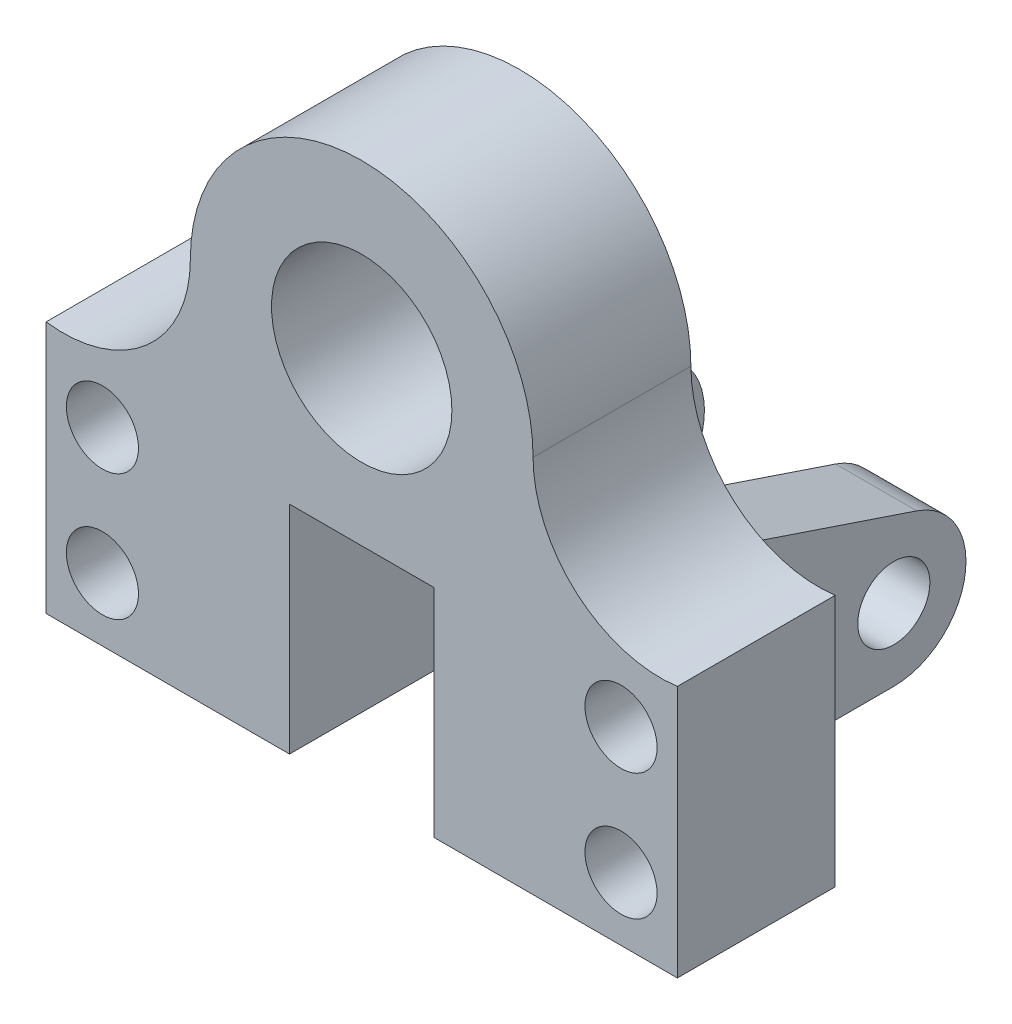
ISO-10303-21;
HEADER;
FILE_DESCRIPTION(('STEP AP214'),'2;1');
FILE_NAME('part.step','',(''),(''),'','','');
FILE_SCHEMA(('AUTOMOTIVE_DESIGN { 1 0 10303 214 1 1 1 1 }'));
ENDSEC;
DATA;
#1=APPLICATION_CONTEXT('core data for automotive mechanical design processes');
#2=APPLICATION_PROTOCOL_DEFINITION('international standard','automotive_design',2000,#1);
#3=PRODUCT_CONTEXT('',#1,'mechanical');
#4=PRODUCT('Part','Part','',(#3));
#5=PRODUCT_RELATED_PRODUCT_CATEGORY('part','',(#4));
#6=PRODUCT_DEFINITION_FORMATION('','',#4);
#7=PRODUCT_DEFINITION_CONTEXT('part definition',#1,'design');
#8=PRODUCT_DEFINITION('design','',#6,#7);
#9=PRODUCT_DEFINITION_SHAPE('','',#8);
#10=(LENGTH_UNIT() NAMED_UNIT(*) SI_UNIT(.MILLI.,.METRE.));
#11=(NAMED_UNIT(*) PLANE_ANGLE_UNIT() SI_UNIT($,.RADIAN.));
#12=(NAMED_UNIT(*) SI_UNIT($,.STERADIAN.) SOLID_ANGLE_UNIT());
#13=UNCERTAINTY_MEASURE_WITH_UNIT(LENGTH_MEASURE(1.E-05),#10,'distance_accuracy_value','');
#14=(GEOMETRIC_REPRESENTATION_CONTEXT(3) GLOBAL_UNCERTAINTY_ASSIGNED_CONTEXT((#13)) GLOBAL_UNIT_ASSIGNED_CONTEXT((#10,
#11,#12)) REPRESENTATION_CONTEXT('',''));
#15=CARTESIAN_POINT('',(0.,0.,0.));
#16=DIRECTION('',(0.,0.,1.));
#17=DIRECTION('',(1.,0.,0.));
#18=AXIS2_PLACEMENT_3D('',#15,#16,#17);
#19=CARTESIAN_POINT('',(-70.,-84.,35.));
#20=DIRECTION('',(0.,1.,0.));
#21=DIRECTION('',(0.,0.,1.));
#22=AXIS2_PLACEMENT_3D('',#19,#20,#21);
#23=PLANE('',#22);
#24=DIRECTION('',(0.,0.,-1.));
#25=VECTOR('',#24,1.);
#26=CARTESIAN_POINT('',(-16.,-84.,35.));
#27=LINE('',#26,#25);
#28=CARTESIAN_POINT('',(-16.,-84.,35.));
#29=VERTEX_POINT('',#28);
#30=CARTESIAN_POINT('',(-16.,-84.,0.));
#31=VERTEX_POINT('',#30);
#32=EDGE_CURVE('E175',#29,#31,#27,.T.);
#33=ORIENTED_EDGE('',*,*,#32,.F.);
#34=DIRECTION('',(1.,0.,0.));
#35=VECTOR('',#34,1.);
#36=CARTESIAN_POINT('',(-70.,-84.,35.));
#37=LINE('',#36,#35);
#38=CARTESIAN_POINT('',(-70.,-84.,35.));
#39=VERTEX_POINT('',#38);
#40=EDGE_CURVE('E189',#39,#29,#37,.T.);
#41=ORIENTED_EDGE('',*,*,#40,.F.);
#42=DIRECTION('',(0.,0.,-1.));
#43=VECTOR('',#42,1.);
#44=CARTESIAN_POINT('',(-70.,-84.,35.));
#45=LINE('',#44,#43);
#46=CARTESIAN_POINT('',(-70.,-84.,0.));
#47=VERTEX_POINT('',#46);
#48=EDGE_CURVE('E231',#39,#47,#45,.T.);
#49=ORIENTED_EDGE('',*,*,#48,.T.);
#50=DIRECTION('',(1.,0.,0.));
#51=VECTOR('',#50,1.);
#52=CARTESIAN_POINT('',(-70.,-84.,0.));
#53=LINE('',#52,#51);
#54=CARTESIAN_POINT('',(-38.,-84.,0.));
#55=VERTEX_POINT('',#54);
#56=EDGE_CURVE('E211',#47,#55,#53,.T.);
#57=ORIENTED_EDGE('',*,*,#56,.T.);
#58=DIRECTION('',(0.,0.,-1.));
#59=VECTOR('',#58,1.);
#60=CARTESIAN_POINT('',(-38.,-84.,0.));
#61=LINE('',#60,#59);
#62=CARTESIAN_POINT('',(-38.,-84.,-45.));
#63=VERTEX_POINT('',#62);
#64=EDGE_CURVE('E292',#55,#63,#61,.T.);
#65=ORIENTED_EDGE('',*,*,#64,.T.);
#66=DIRECTION('',(-1.,0.,0.));
#67=VECTOR('',#66,1.);
#68=CARTESIAN_POINT('',(-20.,-84.,-45.));
#69=LINE('',#68,#67);
#70=CARTESIAN_POINT('',(-20.,-84.,-45.));
#71=VERTEX_POINT('',#70);
#72=EDGE_CURVE('E304',#71,#63,#69,.T.);
#73=ORIENTED_EDGE('',*,*,#72,.F.);
#74=DIRECTION('',(0.,0.,-1.));
#75=VECTOR('',#74,1.);
#76=CARTESIAN_POINT('',(-20.,-84.,0.));
#77=LINE('',#76,#75);
#78=CARTESIAN_POINT('',(-20.,-84.,0.));
#79=VERTEX_POINT('',#78);
#80=EDGE_CURVE('E386',#79,#71,#77,.T.);
#81=ORIENTED_EDGE('',*,*,#80,.F.);
#82=EDGE_CURVE('E214',#79,#31,#53,.T.);
#83=ORIENTED_EDGE('',*,*,#82,.T.);
#84=EDGE_LOOP('',(#33,#41,#49,#57,#65,#73,#81,#83));
#85=FACE_BOUND('',#84,.T.);
#86=ADVANCED_FACE('F41',(#85),#23,.F.);
#87=CARTESIAN_POINT('',(-66.25,0.,0.));
#88=DIRECTION('',(0.,0.,1.));
#89=DIRECTION('',(1.,0.,0.));
#90=AXIS2_PLACEMENT_3D('',#87,#88,#89);
#91=PLANE('',#90);
#92=CARTESIAN_POINT('',(0.,0.,0.));
#93=DIRECTION('',(0.,0.,1.));
#94=DIRECTION('',(1.,0.,0.));
#95=AXIS2_PLACEMENT_3D('',#92,#93,#94);
#96=CIRCLE('',#95,21.);
#97=CARTESIAN_POINT('',(21.,0.,0.));
#98=VERTEX_POINT('',#97);
#99=EDGE_CURVE('E49',#98,#98,#96,.T.);
#100=ORIENTED_EDGE('',*,*,#99,.T.);
#101=EDGE_LOOP('',(#100));
#102=FACE_BOUND('',#101,.T.);
#103=CARTESIAN_POINT('',(-57.5,-70.,0.));
#104=DIRECTION('',(0.,0.,1.));
#105=DIRECTION('',(1.,0.,0.));
#106=AXIS2_PLACEMENT_3D('',#103,#104,#105);
#107=CIRCLE('',#106,8.);
#108=CARTESIAN_POINT('',(-49.5,-70.,0.));
#109=VERTEX_POINT('',#108);
#110=EDGE_CURVE('E356',#109,#109,#107,.T.);
#111=ORIENTED_EDGE('',*,*,#110,.T.);
#112=EDGE_LOOP('',(#111));
#113=FACE_BOUND('',#112,.T.);
#114=CARTESIAN_POINT('',(57.5,-42.,0.));
#115=DIRECTION('',(0.,0.,1.));
#116=DIRECTION('',(1.,0.,0.));
#117=AXIS2_PLACEMENT_3D('',#114,#115,#116);
#118=CIRCLE('',#117,8.00000000000003);
#119=CARTESIAN_POINT('',(65.5,-42.,0.));
#120=VERTEX_POINT('',#119);
#121=EDGE_CURVE('E349',#120,#120,#118,.T.);
#122=ORIENTED_EDGE('',*,*,#121,.T.);
#123=EDGE_LOOP('',(#122));
#124=FACE_BOUND('',#123,.T.);
#125=CARTESIAN_POINT('',(57.5,-70.,0.));
#126=DIRECTION('',(0.,0.,1.));
#127=DIRECTION('',(1.,0.,0.));
#128=AXIS2_PLACEMENT_3D('',#125,#126,#127);
#129=CIRCLE('',#128,8.00000000000001);
#130=CARTESIAN_POINT('',(65.5,-70.,0.));
#131=VERTEX_POINT('',#130);
#132=EDGE_CURVE('E345',#131,#131,#129,.T.);
#133=ORIENTED_EDGE('',*,*,#132,.T.);
#134=EDGE_LOOP('',(#133));
#135=FACE_BOUND('',#134,.T.);
#136=CARTESIAN_POINT('',(-57.5,-42.,0.));
#137=DIRECTION('',(0.,0.,1.));
#138=DIRECTION('',(1.,0.,0.));
#139=AXIS2_PLACEMENT_3D('',#136,#137,#138);
#140=CIRCLE('',#139,8.);
#141=CARTESIAN_POINT('',(-49.5,-42.,0.));
#142=VERTEX_POINT('',#141);
#143=EDGE_CURVE('E365',#142,#142,#140,.T.);
#144=ORIENTED_EDGE('',*,*,#143,.T.);
#145=EDGE_LOOP('',(#144));
#146=FACE_BOUND('',#145,.T.);
#147=DIRECTION('',(0.,-1.,0.));
#148=VECTOR('',#147,1.);
#149=CARTESIAN_POINT('',(16.,-36.,0.));
#150=LINE('',#149,#148);
#151=CARTESIAN_POINT('',(16.,-36.,0.));
#152=VERTEX_POINT('',#151);
#153=CARTESIAN_POINT('',(16.,-84.,0.));
#154=VERTEX_POINT('',#153);
#155=EDGE_CURVE('E169',#152,#154,#150,.T.);
#156=ORIENTED_EDGE('',*,*,#155,.F.);
#157=DIRECTION('',(1.,0.,0.));
#158=VECTOR('',#157,1.);
#159=CARTESIAN_POINT('',(-16.,-36.,0.));
#160=LINE('',#159,#158);
#161=CARTESIAN_POINT('',(-16.,-36.,0.));
#162=VERTEX_POINT('',#161);
#163=EDGE_CURVE('E181',#162,#152,#160,.T.);
#164=ORIENTED_EDGE('',*,*,#163,.F.);
#165=DIRECTION('',(0.,1.,0.));
#166=VECTOR('',#165,1.);
#167=CARTESIAN_POINT('',(-16.,-84.,0.));
#168=LINE('',#167,#166);
#169=EDGE_CURVE('E396',#31,#162,#168,.T.);
#170=ORIENTED_EDGE('',*,*,#169,.F.);
#171=ORIENTED_EDGE('',*,*,#82,.F.);
#172=DIRECTION('',(0.,-1.,0.));
#173=VECTOR('',#172,1.);
#174=CARTESIAN_POINT('',(-20.,-36.,0.));
#175=LINE('',#174,#173);
#176=CARTESIAN_POINT('',(-20.,-36.,0.));
#177=VERTEX_POINT('',#176);
#178=EDGE_CURVE('E395',#177,#79,#175,.T.);
#179=ORIENTED_EDGE('',*,*,#178,.F.);
#180=DIRECTION('',(-1.,0.,0.));
#181=VECTOR('',#180,1.);
#182=CARTESIAN_POINT('',(-20.,-36.,0.));
#183=LINE('',#182,#181);
#184=CARTESIAN_POINT('',(-38.,-36.,0.));
#185=VERTEX_POINT('',#184);
#186=EDGE_CURVE('E62',#177,#185,#183,.T.);
#187=ORIENTED_EDGE('',*,*,#186,.T.);
#188=DIRECTION('',(0.,-1.,0.));
#189=VECTOR('',#188,1.);
#190=CARTESIAN_POINT('',(-38.,-36.,0.));
#191=LINE('',#190,#189);
#192=EDGE_CURVE('E290',#185,#55,#191,.T.);
#193=ORIENTED_EDGE('',*,*,#192,.T.);
#194=ORIENTED_EDGE('',*,*,#56,.F.);
#195=DIRECTION('',(0.,-1.,0.));
#196=VECTOR('',#195,1.);
#197=CARTESIAN_POINT('',(-70.,-28.,0.));
#198=LINE('',#197,#196);
#199=CARTESIAN_POINT('',(-70.,-28.,0.));
#200=VERTEX_POINT('',#199);
#201=EDGE_CURVE('E210',#200,#47,#198,.T.);
#202=ORIENTED_EDGE('',*,*,#201,.F.);
#203=CARTESIAN_POINT('',(-66.25,0.,0.));
#204=DIRECTION('',(0.,0.,-1.));
#205=DIRECTION('',(1.,0.,0.));
#206=AXIS2_PLACEMENT_3D('',#203,#204,#205);
#207=CIRCLE('',#206,28.25);
#208=CARTESIAN_POINT('',(-38.,0.,0.));
#209=VERTEX_POINT('',#208);
#210=EDGE_CURVE('E204',#209,#200,#207,.T.);
#211=ORIENTED_EDGE('',*,*,#210,.F.);
#212=CARTESIAN_POINT('',(0.,0.,0.));
#213=DIRECTION('',(0.,0.,1.));
#214=DIRECTION('',(1.,0.,0.));
#215=AXIS2_PLACEMENT_3D('',#212,#213,#214);
#216=CIRCLE('',#215,38.);
#217=CARTESIAN_POINT('',(38.,0.,0.));
#218=VERTEX_POINT('',#217);
#219=EDGE_CURVE('E219',#218,#209,#216,.T.);
#220=ORIENTED_EDGE('',*,*,#219,.F.);
#221=CARTESIAN_POINT('',(66.25,0.,0.));
#222=DIRECTION('',(0.,0.,-1.));
#223=DIRECTION('',(1.,0.,0.));
#224=AXIS2_PLACEMENT_3D('',#221,#222,#223);
#225=CIRCLE('',#224,28.25);
#226=CARTESIAN_POINT('',(70.,-28.,0.));
#227=VERTEX_POINT('',#226);
#228=EDGE_CURVE('E217',#227,#218,#225,.T.);
#229=ORIENTED_EDGE('',*,*,#228,.F.);
#230=DIRECTION('',(0.,1.,0.));
#231=VECTOR('',#230,1.);
#232=CARTESIAN_POINT('',(70.,-84.,0.));
#233=LINE('',#232,#231);
#234=CARTESIAN_POINT('',(70.,-84.,0.));
#235=VERTEX_POINT('',#234);
#236=EDGE_CURVE('E212',#235,#227,#233,.T.);
#237=ORIENTED_EDGE('',*,*,#236,.F.);
#238=CARTESIAN_POINT('',(38.,-84.,0.));
#239=VERTEX_POINT('',#238);
#240=EDGE_CURVE('E209',#239,#235,#53,.T.);
#241=ORIENTED_EDGE('',*,*,#240,.F.);
#242=DIRECTION('',(0.,-1.,0.));
#243=VECTOR('',#242,1.);
#244=CARTESIAN_POINT('',(38.,-84.,0.));
#245=LINE('',#244,#243);
#246=CARTESIAN_POINT('',(38.,-36.,0.));
#247=VERTEX_POINT('',#246);
#248=EDGE_CURVE('E321',#247,#239,#245,.T.);
#249=ORIENTED_EDGE('',*,*,#248,.F.);
#250=DIRECTION('',(1.,0.,0.));
#251=VECTOR('',#250,1.);
#252=CARTESIAN_POINT('',(20.,-36.,0.));
#253=LINE('',#252,#251);
#254=CARTESIAN_POINT('',(20.,-36.,0.));
#255=VERTEX_POINT('',#254);
#256=EDGE_CURVE('E337',#255,#247,#253,.T.);
#257=ORIENTED_EDGE('',*,*,#256,.F.);
#258=DIRECTION('',(0.,-1.,0.));
#259=VECTOR('',#258,1.);
#260=CARTESIAN_POINT('',(20.,-84.,0.));
#261=LINE('',#260,#259);
#262=CARTESIAN_POINT('',(20.,-84.,0.));
#263=VERTEX_POINT('',#262);
#264=EDGE_CURVE('E326',#255,#263,#261,.T.);
#265=ORIENTED_EDGE('',*,*,#264,.T.);
#266=EDGE_CURVE('E216',#154,#263,#53,.T.);
#267=ORIENTED_EDGE('',*,*,#266,.F.);
#268=EDGE_LOOP('',(#156,#164,#170,#171,#179,#187,#193,#194,#202,#211,#220,#229,#237,#241,#249,
#257,#265,#267));
#269=FACE_BOUND('',#268,.T.);
#270=ADVANCED_FACE('F239',(#102,#113,#124,#135,#146,#269),#91,.F.);
#271=CARTESIAN_POINT('',(-66.25,0.,35.));
#272=DIRECTION('',(0.,0.,1.));
#273=DIRECTION('',(1.,0.,0.));
#274=AXIS2_PLACEMENT_3D('',#271,#272,#273);
#275=PLANE('',#274);
#276=CARTESIAN_POINT('',(-57.5,-70.,35.));
#277=DIRECTION('',(0.,0.,1.));
#278=DIRECTION('',(1.,0.,0.));
#279=AXIS2_PLACEMENT_3D('',#276,#277,#278);
#280=CIRCLE('',#279,8.);
#281=CARTESIAN_POINT('',(-49.5,-70.,35.));
#282=VERTEX_POINT('',#281);
#283=EDGE_CURVE('E355',#282,#282,#280,.T.);
#284=ORIENTED_EDGE('',*,*,#283,.F.);
#285=EDGE_LOOP('',(#284));
#286=FACE_BOUND('',#285,.T.);
#287=CARTESIAN_POINT('',(57.5,-42.,35.));
#288=DIRECTION('',(0.,0.,1.));
#289=DIRECTION('',(1.,0.,0.));
#290=AXIS2_PLACEMENT_3D('',#287,#288,#289);
#291=CIRCLE('',#290,8.00000000000003);
#292=CARTESIAN_POINT('',(65.5,-42.,35.));
#293=VERTEX_POINT('',#292);
#294=EDGE_CURVE('E357',#293,#293,#291,.T.);
#295=ORIENTED_EDGE('',*,*,#294,.F.);
#296=EDGE_LOOP('',(#295));
#297=FACE_BOUND('',#296,.T.);
#298=CARTESIAN_POINT('',(57.5,-70.,35.));
#299=DIRECTION('',(0.,0.,1.));
#300=DIRECTION('',(1.,0.,0.));
#301=AXIS2_PLACEMENT_3D('',#298,#299,#300);
#302=CIRCLE('',#301,8.00000000000001);
#303=CARTESIAN_POINT('',(65.5,-70.,35.));
#304=VERTEX_POINT('',#303);
#305=EDGE_CURVE('E347',#304,#304,#302,.T.);
#306=ORIENTED_EDGE('',*,*,#305,.F.);
#307=EDGE_LOOP('',(#306));
#308=FACE_BOUND('',#307,.T.);
#309=CARTESIAN_POINT('',(-57.5,-42.,35.));
#310=DIRECTION('',(0.,0.,1.));
#311=DIRECTION('',(1.,0.,0.));
#312=AXIS2_PLACEMENT_3D('',#309,#310,#311);
#313=CIRCLE('',#312,8.);
#314=CARTESIAN_POINT('',(-49.5,-42.,35.));
#315=VERTEX_POINT('',#314);
#316=EDGE_CURVE('E352',#315,#315,#313,.T.);
#317=ORIENTED_EDGE('',*,*,#316,.F.);
#318=EDGE_LOOP('',(#317));
#319=FACE_BOUND('',#318,.T.);
#320=CARTESIAN_POINT('',(0.,0.,35.));
#321=DIRECTION('',(0.,0.,1.));
#322=DIRECTION('',(1.,0.,0.));
#323=AXIS2_PLACEMENT_3D('',#320,#321,#322);
#324=CIRCLE('',#323,20.);
#325=CARTESIAN_POINT('',(20.,0.,35.));
#326=VERTEX_POINT('',#325);
#327=EDGE_CURVE('E208',#326,#326,#324,.T.);
#328=ORIENTED_EDGE('',*,*,#327,.F.);
#329=EDGE_LOOP('',(#328));
#330=FACE_BOUND('',#329,.T.);
#331=DIRECTION('',(1.,0.,0.));
#332=VECTOR('',#331,1.);
#333=CARTESIAN_POINT('',(-16.,-36.,35.));
#334=LINE('',#333,#332);
#335=CARTESIAN_POINT('',(-16.,-36.,35.));
#336=VERTEX_POINT('',#335);
#337=CARTESIAN_POINT('',(16.,-36.,35.));
#338=VERTEX_POINT('',#337);
#339=EDGE_CURVE('E171',#336,#338,#334,.T.);
#340=ORIENTED_EDGE('',*,*,#339,.T.);
#341=DIRECTION('',(0.,-1.,0.));
#342=VECTOR('',#341,1.);
#343=CARTESIAN_POINT('',(16.,-36.,35.));
#344=LINE('',#343,#342);
#345=CARTESIAN_POINT('',(16.,-84.,35.));
#346=VERTEX_POINT('',#345);
#347=EDGE_CURVE('E60',#338,#346,#344,.T.);
#348=ORIENTED_EDGE('',*,*,#347,.T.);
#349=CARTESIAN_POINT('',(70.,-84.,35.));
#350=VERTEX_POINT('',#349);
#351=EDGE_CURVE('E178',#346,#350,#37,.T.);
#352=ORIENTED_EDGE('',*,*,#351,.T.);
#353=DIRECTION('',(0.,1.,0.));
#354=VECTOR('',#353,1.);
#355=CARTESIAN_POINT('',(70.,-84.,35.));
#356=LINE('',#355,#354);
#357=CARTESIAN_POINT('',(70.,-28.,35.));
#358=VERTEX_POINT('',#357);
#359=EDGE_CURVE('E193',#350,#358,#356,.T.);
#360=ORIENTED_EDGE('',*,*,#359,.T.);
#361=CARTESIAN_POINT('',(66.25,0.,35.));
#362=DIRECTION('',(0.,0.,-1.));
#363=DIRECTION('',(1.,0.,0.));
#364=AXIS2_PLACEMENT_3D('',#361,#362,#363);
#365=CIRCLE('',#364,28.25);
#366=CARTESIAN_POINT('',(38.,0.,35.));
#367=VERTEX_POINT('',#366);
#368=EDGE_CURVE('E200',#358,#367,#365,.T.);
#369=ORIENTED_EDGE('',*,*,#368,.T.);
#370=CARTESIAN_POINT('',(0.,0.,35.));
#371=DIRECTION('',(0.,0.,1.));
#372=DIRECTION('',(1.,0.,0.));
#373=AXIS2_PLACEMENT_3D('',#370,#371,#372);
#374=CIRCLE('',#373,38.);
#375=CARTESIAN_POINT('',(-38.,0.,35.));
#376=VERTEX_POINT('',#375);
#377=EDGE_CURVE('E203',#367,#376,#374,.T.);
#378=ORIENTED_EDGE('',*,*,#377,.T.);
#379=CARTESIAN_POINT('',(-66.25,0.,35.));
#380=DIRECTION('',(0.,0.,-1.));
#381=DIRECTION('',(1.,0.,0.));
#382=AXIS2_PLACEMENT_3D('',#379,#380,#381);
#383=CIRCLE('',#382,28.25);
#384=CARTESIAN_POINT('',(-70.,-28.,35.));
#385=VERTEX_POINT('',#384);
#386=EDGE_CURVE('E192',#376,#385,#383,.T.);
#387=ORIENTED_EDGE('',*,*,#386,.T.);
#388=DIRECTION('',(0.,-1.,0.));
#389=VECTOR('',#388,1.);
#390=CARTESIAN_POINT('',(-70.,-28.,35.));
#391=LINE('',#390,#389);
#392=EDGE_CURVE('E187',#385,#39,#391,.T.);
#393=ORIENTED_EDGE('',*,*,#392,.T.);
#394=ORIENTED_EDGE('',*,*,#40,.T.);
#395=DIRECTION('',(0.,1.,0.));
#396=VECTOR('',#395,1.);
#397=CARTESIAN_POINT('',(-16.,-84.,35.));
#398=LINE('',#397,#396);
#399=EDGE_CURVE('E185',#29,#336,#398,.T.);
#400=ORIENTED_EDGE('',*,*,#399,.T.);
#401=EDGE_LOOP('',(#340,#348,#352,#360,#369,#378,#387,#393,#394,#400));
#402=FACE_BOUND('',#401,.T.);
#403=ADVANCED_FACE('F180',(#286,#297,#308,#319,#330,#402),#275,.T.);
#404=CARTESIAN_POINT('',(-66.25,0.,35.));
#405=DIRECTION('',(0.,0.,-1.));
#406=DIRECTION('',(-1.,0.,0.));
#407=AXIS2_PLACEMENT_3D('',#404,#405,#406);
#408=CYLINDRICAL_SURFACE('',#407,28.25);
#409=ORIENTED_EDGE('',*,*,#210,.T.);
#410=DIRECTION('',(0.,0.,-1.));
#411=VECTOR('',#410,1.);
#412=CARTESIAN_POINT('',(-70.,-28.,35.));
#413=LINE('',#412,#411);
#414=EDGE_CURVE('E232',#385,#200,#413,.T.);
#415=ORIENTED_EDGE('',*,*,#414,.F.);
#416=ORIENTED_EDGE('',*,*,#386,.F.);
#417=DIRECTION('',(0.,0.,-1.));
#418=VECTOR('',#417,1.);
#419=CARTESIAN_POINT('',(-38.,0.,35.));
#420=LINE('',#419,#418);
#421=EDGE_CURVE('E201',#376,#209,#420,.T.);
#422=ORIENTED_EDGE('',*,*,#421,.T.);
#423=EDGE_LOOP('',(#409,#415,#416,#422));
#424=FACE_BOUND('',#423,.T.);
#425=ADVANCED_FACE('F274',(#424),#408,.F.);
#426=CARTESIAN_POINT('',(-70.,-28.,35.));
#427=DIRECTION('',(1.,0.,0.));
#428=DIRECTION('',(0.,1.,0.));
#429=AXIS2_PLACEMENT_3D('',#426,#427,#428);
#430=PLANE('',#429);
#431=ORIENTED_EDGE('',*,*,#201,.T.);
#432=ORIENTED_EDGE('',*,*,#48,.F.);
#433=ORIENTED_EDGE('',*,*,#392,.F.);
#434=ORIENTED_EDGE('',*,*,#414,.T.);
#435=EDGE_LOOP('',(#431,#432,#433,#434));
#436=FACE_BOUND('',#435,.T.);
#437=ADVANCED_FACE('F270',(#436),#430,.F.);
#438=ORIENTED_EDGE('',*,*,#351,.F.);
#439=DIRECTION('',(0.,0.,-1.));
#440=VECTOR('',#439,1.);
#441=CARTESIAN_POINT('',(16.,-84.,35.));
#442=LINE('',#441,#440);
#443=EDGE_CURVE('E164',#346,#154,#442,.T.);
#444=ORIENTED_EDGE('',*,*,#443,.T.);
#445=ORIENTED_EDGE('',*,*,#266,.T.);
#446=DIRECTION('',(0.,0.,-1.));
#447=VECTOR('',#446,1.);
#448=CARTESIAN_POINT('',(20.,-84.,0.));
#449=LINE('',#448,#447);
#450=CARTESIAN_POINT('',(20.,-84.,-45.));
#451=VERTEX_POINT('',#450);
#452=EDGE_CURVE('E320',#263,#451,#449,.T.);
#453=ORIENTED_EDGE('',*,*,#452,.T.);
#454=DIRECTION('',(1.,0.,0.));
#455=VECTOR('',#454,1.);
#456=CARTESIAN_POINT('',(20.,-84.,-45.));
#457=LINE('',#456,#455);
#458=CARTESIAN_POINT('',(38.,-84.,-45.));
#459=VERTEX_POINT('',#458);
#460=EDGE_CURVE('E328',#451,#459,#457,.T.);
#461=ORIENTED_EDGE('',*,*,#460,.T.);
#462=DIRECTION('',(0.,0.,-1.));
#463=VECTOR('',#462,1.);
#464=CARTESIAN_POINT('',(38.,-84.,0.));
#465=LINE('',#464,#463);
#466=EDGE_CURVE('E314',#239,#459,#465,.T.);
#467=ORIENTED_EDGE('',*,*,#466,.F.);
#468=ORIENTED_EDGE('',*,*,#240,.T.);
#469=DIRECTION('',(0.,0.,-1.));
#470=VECTOR('',#469,1.);
#471=CARTESIAN_POINT('',(70.,-84.,35.));
#472=LINE('',#471,#470);
#473=EDGE_CURVE('E190',#350,#235,#472,.T.);
#474=ORIENTED_EDGE('',*,*,#473,.F.);
#475=EDGE_LOOP('',(#438,#444,#445,#453,#461,#467,#468,#474));
#476=FACE_BOUND('',#475,.T.);
#477=ADVANCED_FACE('F183',(#476),#23,.F.);
#478=CARTESIAN_POINT('',(70.,-84.,35.));
#479=DIRECTION('',(-1.,0.,0.));
#480=DIRECTION('',(0.,0.,1.));
#481=AXIS2_PLACEMENT_3D('',#478,#479,#480);
#482=PLANE('',#481);
#483=ORIENTED_EDGE('',*,*,#236,.T.);
#484=DIRECTION('',(0.,0.,-1.));
#485=VECTOR('',#484,1.);
#486=CARTESIAN_POINT('',(70.,-28.,35.));
#487=LINE('',#486,#485);
#488=EDGE_CURVE('E230',#358,#227,#487,.T.);
#489=ORIENTED_EDGE('',*,*,#488,.F.);
#490=ORIENTED_EDGE('',*,*,#359,.F.);
#491=ORIENTED_EDGE('',*,*,#473,.T.);
#492=EDGE_LOOP('',(#483,#489,#490,#491));
#493=FACE_BOUND('',#492,.T.);
#494=ADVANCED_FACE('F266',(#493),#482,.F.);
#495=CARTESIAN_POINT('',(66.25,0.,35.));
#496=DIRECTION('',(0.,0.,-1.));
#497=DIRECTION('',(-1.,0.,0.));
#498=AXIS2_PLACEMENT_3D('',#495,#496,#497);
#499=CYLINDRICAL_SURFACE('',#498,28.25);
#500=ORIENTED_EDGE('',*,*,#228,.T.);
#501=DIRECTION('',(0.,0.,-1.));
#502=VECTOR('',#501,1.);
#503=CARTESIAN_POINT('',(38.,0.,35.));
#504=LINE('',#503,#502);
#505=EDGE_CURVE('E221',#367,#218,#504,.T.);
#506=ORIENTED_EDGE('',*,*,#505,.F.);
#507=ORIENTED_EDGE('',*,*,#368,.F.);
#508=ORIENTED_EDGE('',*,*,#488,.T.);
#509=EDGE_LOOP('',(#500,#506,#507,#508));
#510=FACE_BOUND('',#509,.T.);
#511=ADVANCED_FACE('F275',(#510),#499,.F.);
#512=CARTESIAN_POINT('',(0.,0.,35.));
#513=DIRECTION('',(0.,0.,-1.));
#514=DIRECTION('',(-1.,0.,0.));
#515=AXIS2_PLACEMENT_3D('',#512,#513,#514);
#516=CYLINDRICAL_SURFACE('',#515,38.);
#517=ORIENTED_EDGE('',*,*,#219,.T.);
#518=ORIENTED_EDGE('',*,*,#421,.F.);
#519=ORIENTED_EDGE('',*,*,#377,.F.);
#520=ORIENTED_EDGE('',*,*,#505,.T.);
#521=EDGE_LOOP('',(#517,#518,#519,#520));
#522=FACE_BOUND('',#521,.T.);
#523=ADVANCED_FACE('F378',(#522),#516,.T.);
#524=CARTESIAN_POINT('',(0.,0.,0.));
#525=DIRECTION('',(0.,0.,1.));
#526=DIRECTION('',(1.,0.,0.));
#527=AXIS2_PLACEMENT_3D('',#524,#525,#526);
#528=CYLINDRICAL_SURFACE('',#527,20.);
#529=CARTESIAN_POINT('',(0.,0.,1.00000000000003));
#530=DIRECTION('',(0.,0.,1.));
#531=DIRECTION('',(1.,0.,0.));
#532=AXIS2_PLACEMENT_3D('',#529,#530,#531);
#533=CIRCLE('',#532,20.);
#534=CARTESIAN_POINT('',(20.,0.,1.00000000000003));
#535=VERTEX_POINT('',#534);
#536=EDGE_CURVE('E11',#535,#535,#533,.F.);
#537=ORIENTED_EDGE('',*,*,#536,.T.);
#538=EDGE_LOOP('',(#537));
#539=FACE_BOUND('',#538,.T.);
#540=ORIENTED_EDGE('',*,*,#327,.T.);
#541=EDGE_LOOP('',(#540));
#542=FACE_BOUND('',#541,.T.);
#543=ADVANCED_FACE('F472',(#539,#542),#528,.F.);
#544=CARTESIAN_POINT('',(-57.5,-42.,0.));
#545=DIRECTION('',(0.,0.,1.));
#546=DIRECTION('',(1.,0.,0.));
#547=AXIS2_PLACEMENT_3D('',#544,#545,#546);
#548=CYLINDRICAL_SURFACE('',#547,8.);
#549=ORIENTED_EDGE('',*,*,#143,.F.);
#550=EDGE_LOOP('',(#549));
#551=FACE_BOUND('',#550,.T.);
#552=ORIENTED_EDGE('',*,*,#316,.T.);
#553=EDGE_LOOP('',(#552));
#554=FACE_BOUND('',#553,.T.);
#555=ADVANCED_FACE('F464',(#551,#554),#548,.F.);
#556=CARTESIAN_POINT('',(57.5,-70.,0.));
#557=DIRECTION('',(0.,0.,1.));
#558=DIRECTION('',(1.,0.,0.));
#559=AXIS2_PLACEMENT_3D('',#556,#557,#558);
#560=CYLINDRICAL_SURFACE('',#559,8.00000000000001);
#561=ORIENTED_EDGE('',*,*,#132,.F.);
#562=EDGE_LOOP('',(#561));
#563=FACE_BOUND('',#562,.T.);
#564=ORIENTED_EDGE('',*,*,#305,.T.);
#565=EDGE_LOOP('',(#564));
#566=FACE_BOUND('',#565,.T.);
#567=ADVANCED_FACE('F465',(#563,#566),#560,.F.);
#568=CARTESIAN_POINT('',(57.5,-42.,0.));
#569=DIRECTION('',(0.,0.,1.));
#570=DIRECTION('',(1.,0.,0.));
#571=AXIS2_PLACEMENT_3D('',#568,#569,#570);
#572=CYLINDRICAL_SURFACE('',#571,8.00000000000003);
#573=ORIENTED_EDGE('',*,*,#121,.F.);
#574=EDGE_LOOP('',(#573));
#575=FACE_BOUND('',#574,.T.);
#576=ORIENTED_EDGE('',*,*,#294,.T.);
#577=EDGE_LOOP('',(#576));
#578=FACE_BOUND('',#577,.T.);
#579=ADVANCED_FACE('F457',(#575,#578),#572,.F.);
#580=CARTESIAN_POINT('',(-57.5,-70.,0.));
#581=DIRECTION('',(0.,0.,1.));
#582=DIRECTION('',(1.,0.,0.));
#583=AXIS2_PLACEMENT_3D('',#580,#581,#582);
#584=CYLINDRICAL_SURFACE('',#583,8.);
#585=ORIENTED_EDGE('',*,*,#110,.F.);
#586=EDGE_LOOP('',(#585));
#587=FACE_BOUND('',#586,.T.);
#588=ORIENTED_EDGE('',*,*,#283,.T.);
#589=EDGE_LOOP('',(#588));
#590=FACE_BOUND('',#589,.T.);
#591=ADVANCED_FACE('F449',(#587,#590),#584,.F.);
#592=CARTESIAN_POINT('',(20.,-36.,0.));
#593=DIRECTION('',(0.,0.947916643853816,-0.318518502296047));
#594=DIRECTION('',(0.,0.318518502296047,0.947916643853816));
#595=AXIS2_PLACEMENT_3D('',#592,#593,#594);
#596=PLANE('',#595);
#597=DIRECTION('',(0.,0.318518502296047,0.947916643853816));
#598=VECTOR('',#597,1.);
#599=CARTESIAN_POINT('',(38.,-36.,0.));
#600=LINE('',#599,#598);
#601=CARTESIAN_POINT('',(38.,-52.8333336983389,-50.0962960367368));
#602=VERTEX_POINT('',#601);
#603=EDGE_CURVE('E333',#602,#247,#600,.T.);
#604=ORIENTED_EDGE('',*,*,#603,.F.);
#605=DIRECTION('',(1.,0.,0.));
#606=VECTOR('',#605,1.);
#607=CARTESIAN_POINT('',(20.,-52.8333336983389,-50.0962960367368));
#608=LINE('',#607,#606);
#609=CARTESIAN_POINT('',(20.,-52.8333336983389,-50.0962960367368));
#610=VERTEX_POINT('',#609);
#611=EDGE_CURVE('E343',#610,#602,#608,.T.);
#612=ORIENTED_EDGE('',*,*,#611,.F.);
#613=DIRECTION('',(0.,0.318518502296047,0.947916643853816));
#614=VECTOR('',#613,1.);
#615=CARTESIAN_POINT('',(20.,-36.,0.));
#616=LINE('',#615,#614);
#617=EDGE_CURVE('E322',#610,#255,#616,.T.);
#618=ORIENTED_EDGE('',*,*,#617,.T.);
#619=ORIENTED_EDGE('',*,*,#256,.T.);
#620=EDGE_LOOP('',(#604,#612,#618,#619));
#621=FACE_BOUND('',#620,.T.);
#622=ADVANCED_FACE('F450',(#621),#596,.T.);
#623=CARTESIAN_POINT('',(20.,-68.,-45.));
#624=DIRECTION('',(1.,0.,0.));
#625=DIRECTION('',(0.,0.,-1.));
#626=AXIS2_PLACEMENT_3D('',#623,#624,#625);
#627=CYLINDRICAL_SURFACE('',#626,16.);
#628=CARTESIAN_POINT('',(38.,-68.,-45.));
#629=DIRECTION('',(1.,0.,0.));
#630=DIRECTION('',(0.,0.,-1.));
#631=AXIS2_PLACEMENT_3D('',#628,#629,#630);
#632=CIRCLE('',#631,16.);
#633=EDGE_CURVE('E335',#459,#602,#632,.T.);
#634=ORIENTED_EDGE('',*,*,#633,.F.);
#635=ORIENTED_EDGE('',*,*,#460,.F.);
#636=CARTESIAN_POINT('',(20.,-68.,-45.));
#637=DIRECTION('',(1.,0.,0.));
#638=DIRECTION('',(0.,0.,-1.));
#639=AXIS2_PLACEMENT_3D('',#636,#637,#638);
#640=CIRCLE('',#639,16.);
#641=EDGE_CURVE('E319',#451,#610,#640,.T.);
#642=ORIENTED_EDGE('',*,*,#641,.T.);
#643=ORIENTED_EDGE('',*,*,#611,.T.);
#644=EDGE_LOOP('',(#634,#635,#642,#643));
#645=FACE_BOUND('',#644,.T.);
#646=ADVANCED_FACE('F445',(#645),#627,.T.);
#647=CARTESIAN_POINT('',(20.,-68.,-45.));
#648=DIRECTION('',(1.,0.,0.));
#649=DIRECTION('',(0.,0.,-1.));
#650=AXIS2_PLACEMENT_3D('',#647,#648,#649);
#651=PLANE('',#650);
#652=CARTESIAN_POINT('',(20.,-68.,-45.));
#653=DIRECTION('',(1.,0.,0.));
#654=DIRECTION('',(0.,0.,-1.));
#655=AXIS2_PLACEMENT_3D('',#652,#653,#654);
#656=CIRCLE('',#655,8.);
#657=CARTESIAN_POINT('',(20.,-68.,-53.));
#658=VERTEX_POINT('',#657);
#659=EDGE_CURVE('E313',#658,#658,#656,.T.);
#660=ORIENTED_EDGE('',*,*,#659,.T.);
#661=EDGE_LOOP('',(#660));
#662=FACE_BOUND('',#661,.T.);
#663=ORIENTED_EDGE('',*,*,#452,.F.);
#664=ORIENTED_EDGE('',*,*,#264,.F.);
#665=ORIENTED_EDGE('',*,*,#617,.F.);
#666=ORIENTED_EDGE('',*,*,#641,.F.);
#667=EDGE_LOOP('',(#663,#664,#665,#666));
#668=FACE_BOUND('',#667,.T.);
#669=ADVANCED_FACE('F437',(#662,#668),#651,.F.);
#670=CARTESIAN_POINT('',(38.,-68.,-45.));
#671=DIRECTION('',(1.,0.,0.));
#672=DIRECTION('',(0.,0.,-1.));
#673=AXIS2_PLACEMENT_3D('',#670,#671,#672);
#674=PLANE('',#673);
#675=CARTESIAN_POINT('',(38.,-68.,-45.));
#676=DIRECTION('',(1.,0.,0.));
#677=DIRECTION('',(0.,0.,-1.));
#678=AXIS2_PLACEMENT_3D('',#675,#676,#677);
#679=CIRCLE('',#678,8.);
#680=CARTESIAN_POINT('',(38.,-68.,-53.));
#681=VERTEX_POINT('',#680);
#682=EDGE_CURVE('E309',#681,#681,#679,.T.);
#683=ORIENTED_EDGE('',*,*,#682,.F.);
#684=EDGE_LOOP('',(#683));
#685=FACE_BOUND('',#684,.T.);
#686=ORIENTED_EDGE('',*,*,#466,.T.);
#687=ORIENTED_EDGE('',*,*,#633,.T.);
#688=ORIENTED_EDGE('',*,*,#603,.T.);
#689=ORIENTED_EDGE('',*,*,#248,.T.);
#690=EDGE_LOOP('',(#686,#687,#688,#689));
#691=FACE_BOUND('',#690,.T.);
#692=ADVANCED_FACE('F443',(#685,#691),#674,.T.);
#693=CARTESIAN_POINT('',(20.,-68.,-45.));
#694=DIRECTION('',(1.,0.,0.));
#695=DIRECTION('',(0.,0.,-1.));
#696=AXIS2_PLACEMENT_3D('',#693,#694,#695);
#697=CYLINDRICAL_SURFACE('',#696,8.);
#698=ORIENTED_EDGE('',*,*,#659,.F.);
#699=EDGE_LOOP('',(#698));
#700=FACE_BOUND('',#699,.T.);
#701=ORIENTED_EDGE('',*,*,#682,.T.);
#702=EDGE_LOOP('',(#701));
#703=FACE_BOUND('',#702,.T.);
#704=ADVANCED_FACE('F548',(#700,#703),#697,.F.);
#705=CARTESIAN_POINT('',(-20.,-68.,-45.));
#706=DIRECTION('',(1.,0.,0.));
#707=DIRECTION('',(0.,0.,-1.));
#708=AXIS2_PLACEMENT_3D('',#705,#706,#707);
#709=PLANE('',#708);
#710=DIRECTION('',(0.,0.318518502296047,0.947916643853816));
#711=VECTOR('',#710,1.);
#712=CARTESIAN_POINT('',(-20.,-52.8333336983389,-50.0962960367368));
#713=LINE('',#712,#711);
#714=CARTESIAN_POINT('',(-20.,-52.8333336983389,-50.0962960367368));
#715=VERTEX_POINT('',#714);
#716=EDGE_CURVE('E301',#715,#177,#713,.T.);
#717=ORIENTED_EDGE('',*,*,#716,.T.);
#718=ORIENTED_EDGE('',*,*,#178,.T.);
#719=ORIENTED_EDGE('',*,*,#80,.T.);
#720=CARTESIAN_POINT('',(-20.,-68.,-45.));
#721=DIRECTION('',(1.,0.,0.));
#722=DIRECTION('',(0.,0.,-1.));
#723=AXIS2_PLACEMENT_3D('',#720,#721,#722);
#724=CIRCLE('',#723,16.);
#725=EDGE_CURVE('E308',#71,#715,#724,.T.);
#726=ORIENTED_EDGE('',*,*,#725,.T.);
#727=EDGE_LOOP('',(#717,#718,#719,#726));
#728=FACE_BOUND('',#727,.T.);
#729=CARTESIAN_POINT('',(-20.,-68.,-45.));
#730=DIRECTION('',(1.,0.,0.));
#731=DIRECTION('',(0.,0.,-1.));
#732=AXIS2_PLACEMENT_3D('',#729,#730,#731);
#733=CIRCLE('',#732,8.);
#734=CARTESIAN_POINT('',(-20.,-68.,-53.));
#735=VERTEX_POINT('',#734);
#736=EDGE_CURVE('E298',#735,#735,#733,.T.);
#737=ORIENTED_EDGE('',*,*,#736,.F.);
#738=EDGE_LOOP('',(#737));
#739=FACE_BOUND('',#738,.T.);
#740=ADVANCED_FACE('F398',(#728,#739),#709,.T.);
#741=CARTESIAN_POINT('',(-38.,-68.,-45.));
#742=DIRECTION('',(1.,0.,0.));
#743=DIRECTION('',(0.,0.,-1.));
#744=AXIS2_PLACEMENT_3D('',#741,#742,#743);
#745=PLANE('',#744);
#746=DIRECTION('',(0.,0.318518502296047,0.947916643853816));
#747=VECTOR('',#746,1.);
#748=CARTESIAN_POINT('',(-38.,-52.8333336983389,-50.0962960367368));
#749=LINE('',#748,#747);
#750=CARTESIAN_POINT('',(-38.,-52.8333336983389,-50.0962960367368));
#751=VERTEX_POINT('',#750);
#752=EDGE_CURVE('E295',#751,#185,#749,.T.);
#753=ORIENTED_EDGE('',*,*,#752,.F.);
#754=CARTESIAN_POINT('',(-38.,-68.,-45.));
#755=DIRECTION('',(1.,0.,0.));
#756=DIRECTION('',(0.,0.,-1.));
#757=AXIS2_PLACEMENT_3D('',#754,#755,#756);
#758=CIRCLE('',#757,16.);
#759=EDGE_CURVE('E294',#63,#751,#758,.T.);
#760=ORIENTED_EDGE('',*,*,#759,.F.);
#761=ORIENTED_EDGE('',*,*,#64,.F.);
#762=ORIENTED_EDGE('',*,*,#192,.F.);
#763=EDGE_LOOP('',(#753,#760,#761,#762));
#764=FACE_BOUND('',#763,.T.);
#765=CARTESIAN_POINT('',(-38.,-68.,-45.));
#766=DIRECTION('',(1.,0.,0.));
#767=DIRECTION('',(0.,0.,-1.));
#768=AXIS2_PLACEMENT_3D('',#765,#766,#767);
#769=CIRCLE('',#768,8.);
#770=CARTESIAN_POINT('',(-38.,-68.,-53.));
#771=VERTEX_POINT('',#770);
#772=EDGE_CURVE('E416',#771,#771,#769,.T.);
#773=ORIENTED_EDGE('',*,*,#772,.T.);
#774=EDGE_LOOP('',(#773));
#775=FACE_BOUND('',#774,.T.);
#776=ADVANCED_FACE('F415',(#764,#775),#745,.F.);
#777=CARTESIAN_POINT('',(-20.,-52.8333336983389,-50.0962960367368));
#778=DIRECTION('',(0.,-0.947916643853816,0.318518502296047));
#779=DIRECTION('',(0.,-0.318518502296047,-0.947916643853816));
#780=AXIS2_PLACEMENT_3D('',#777,#778,#779);
#781=PLANE('',#780);
#782=ORIENTED_EDGE('',*,*,#752,.T.);
#783=ORIENTED_EDGE('',*,*,#186,.F.);
#784=ORIENTED_EDGE('',*,*,#716,.F.);
#785=DIRECTION('',(-1.,0.,0.));
#786=VECTOR('',#785,1.);
#787=CARTESIAN_POINT('',(-20.,-52.8333336983389,-50.0962960367368));
#788=LINE('',#787,#786);
#789=EDGE_CURVE('E305',#715,#751,#788,.T.);
#790=ORIENTED_EDGE('',*,*,#789,.T.);
#791=EDGE_LOOP('',(#782,#783,#784,#790));
#792=FACE_BOUND('',#791,.T.);
#793=ADVANCED_FACE('F411',(#792),#781,.F.);
#794=CARTESIAN_POINT('',(-20.,-68.,-45.));
#795=DIRECTION('',(-1.,0.,0.));
#796=DIRECTION('',(0.,0.,1.));
#797=AXIS2_PLACEMENT_3D('',#794,#795,#796);
#798=CYLINDRICAL_SURFACE('',#797,16.);
#799=ORIENTED_EDGE('',*,*,#759,.T.);
#800=ORIENTED_EDGE('',*,*,#789,.F.);
#801=ORIENTED_EDGE('',*,*,#725,.F.);
#802=ORIENTED_EDGE('',*,*,#72,.T.);
#803=EDGE_LOOP('',(#799,#800,#801,#802));
#804=FACE_BOUND('',#803,.T.);
#805=ADVANCED_FACE('F406',(#804),#798,.T.);
#806=CARTESIAN_POINT('',(-20.,-68.,-45.));
#807=DIRECTION('',(-1.,0.,0.));
#808=DIRECTION('',(0.,0.,1.));
#809=AXIS2_PLACEMENT_3D('',#806,#807,#808);
#810=CYLINDRICAL_SURFACE('',#809,8.);
#811=ORIENTED_EDGE('',*,*,#736,.T.);
#812=EDGE_LOOP('',(#811));
#813=FACE_BOUND('',#812,.T.);
#814=ORIENTED_EDGE('',*,*,#772,.F.);
#815=EDGE_LOOP('',(#814));
#816=FACE_BOUND('',#815,.T.);
#817=ADVANCED_FACE('F582',(#813,#816),#810,.F.);
#818=CARTESIAN_POINT('',(16.,-36.,35.));
#819=DIRECTION('',(1.,0.,0.));
#820=DIRECTION('',(0.,0.,-1.));
#821=AXIS2_PLACEMENT_3D('',#818,#819,#820);
#822=PLANE('',#821);
#823=ORIENTED_EDGE('',*,*,#155,.T.);
#824=ORIENTED_EDGE('',*,*,#443,.F.);
#825=ORIENTED_EDGE('',*,*,#347,.F.);
#826=DIRECTION('',(0.,0.,-1.));
#827=VECTOR('',#826,1.);
#828=CARTESIAN_POINT('',(16.,-36.,35.));
#829=LINE('',#828,#827);
#830=EDGE_CURVE('E419',#338,#152,#829,.T.);
#831=ORIENTED_EDGE('',*,*,#830,.T.);
#832=EDGE_LOOP('',(#823,#824,#825,#831));
#833=FACE_BOUND('',#832,.T.);
#834=ADVANCED_FACE('F167',(#833),#822,.F.);
#835=CARTESIAN_POINT('',(-16.,-36.,35.));
#836=DIRECTION('',(0.,1.,0.));
#837=DIRECTION('',(0.,0.,1.));
#838=AXIS2_PLACEMENT_3D('',#835,#836,#837);
#839=PLANE('',#838);
#840=ORIENTED_EDGE('',*,*,#163,.T.);
#841=ORIENTED_EDGE('',*,*,#830,.F.);
#842=ORIENTED_EDGE('',*,*,#339,.F.);
#843=DIRECTION('',(0.,0.,-1.));
#844=VECTOR('',#843,1.);
#845=CARTESIAN_POINT('',(-16.,-36.,35.));
#846=LINE('',#845,#844);
#847=EDGE_CURVE('E421',#336,#162,#846,.T.);
#848=ORIENTED_EDGE('',*,*,#847,.T.);
#849=EDGE_LOOP('',(#840,#841,#842,#848));
#850=FACE_BOUND('',#849,.T.);
#851=ADVANCED_FACE('F247',(#850),#839,.F.);
#852=CARTESIAN_POINT('',(-16.,-84.,35.));
#853=DIRECTION('',(-1.,0.,0.));
#854=DIRECTION('',(0.,-1.,0.));
#855=AXIS2_PLACEMENT_3D('',#852,#853,#854);
#856=PLANE('',#855);
#857=ORIENTED_EDGE('',*,*,#169,.T.);
#858=ORIENTED_EDGE('',*,*,#847,.F.);
#859=ORIENTED_EDGE('',*,*,#399,.F.);
#860=ORIENTED_EDGE('',*,*,#32,.T.);
#861=EDGE_LOOP('',(#857,#858,#859,#860));
#862=FACE_BOUND('',#861,.T.);
#863=ADVANCED_FACE('F241',(#862),#856,.F.);
#864=CARTESIAN_POINT('',(0.,0.,0.));
#865=DIRECTION('',(0.,0.,-1.));
#866=DIRECTION('',(-1.,0.,0.));
#867=AXIS2_PLACEMENT_3D('',#864,#865,#866);
#868=CONICAL_SURFACE('',#867,21.,0.785398163397455);
#869=ORIENTED_EDGE('',*,*,#536,.F.);
#870=EDGE_LOOP('',(#869));
#871=FACE_BOUND('',#870,.T.);
#872=ORIENTED_EDGE('',*,*,#99,.F.);
#873=EDGE_LOOP('',(#872));
#874=FACE_BOUND('',#873,.T.);
#875=ADVANCED_FACE('F42',(#871,#874),#868,.F.);
#876=CLOSED_SHELL('',(#86,#270,#403,#425,#437,#477,#494,#511,#523,#543,#555,#567,#579,#591,#622,
#646,#669,#692,#704,#740,#776,#793,#805,#817,#834,#851,#863,#875));
#877=MANIFOLD_SOLID_BREP('B2',#876);
#878=ADVANCED_BREP_SHAPE_REPRESENTATION('',(#18,#877),#14);
#879=SHAPE_DEFINITION_REPRESENTATION(#9,#878);
ENDSEC;
END-ISO-10303-21;
